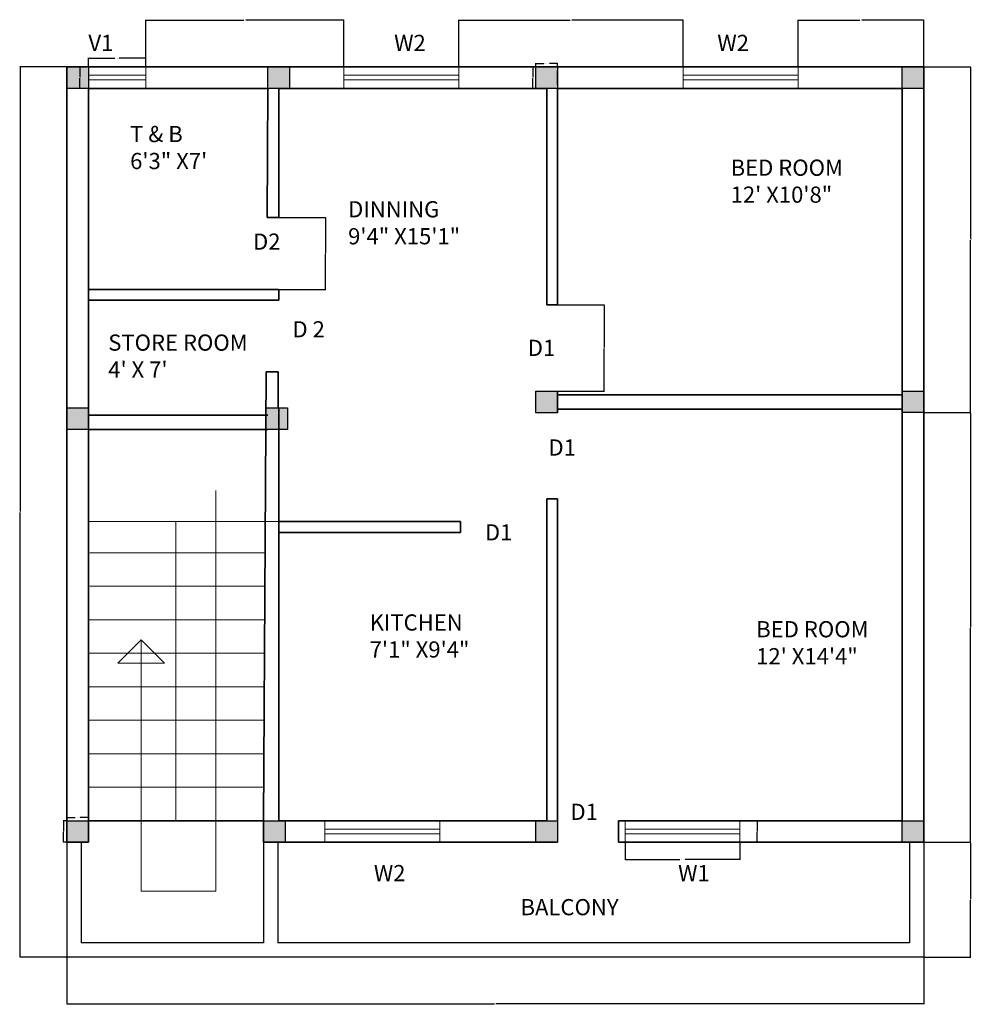
# Model space of a CAD drawing. Units: inches. Extents: x 3504 to 4623, y 2365 to 3357.
# Tile 1 of 5: x 3508 to 3905, y 2372 to 2783. Entities that reach past the tile are written whole.
import ezdxf

# ---------------------------------------------------------------- set-up
doc = ezdxf.new("R2010")
doc.units = ezdxf.units.IN
for name, color, linetype, lineweight in [('A-ANNO-DIMS', 2, 'Continuous', 18), ('A-ANNO-SYMB', 150, 'Continuous', 18), ('A-ANNO-TEXT', 7, 'Continuous', 18), ('A-AREA-IDEN', 7, 'Continuous', 18), ('A-FLOR-HRAL', 7, 'Continuous', 25), ('A-FLOR-STRS', 7, 'Continuous', 18), ('A-GLAZ', 4, 'Continuous', 18), ('A-WALL', 7, 'Continuous', 35)]:
    doc.layers.add(name, color=color, linetype=linetype, lineweight=lineweight)
doc.layers.add('S-COLS', color=244, linetype='Continuous', lineweight=30, true_color=0x991b1e)
doc.layers.add('S-COLS-PATT', color=244, linetype='Continuous', lineweight=13, true_color=0x991b1e)
doc.styles.get("Standard").update_dxf_attribs({"font": 'arial.ttf'})
doc.dimstyles.get("Standard").update_dxf_attribs({"dimtxt": 0.18, "dimasz": 0.18, "dimexe": 0.18, "dimexo": 0.0625, "dimgap": 0.09, "dimtad": 0, "dimtih": 1, "dimtoh": 1, "dimdec": 4, "dimzin": 0, "dimdsep": 46, "dimtxsty": 'Standard', "dimcen": 0.09, "dimadec": 0, "dimazin": 0, "dimtfac": 1, "dimtdec": 4, "dimtofl": 0, "dimtmove": 0, "dimatfit": 3, "dimfxl": 1, "dimtolj": 1, "dimtzin": 0, "dimarcsym": 0})

# ---------------------------------------------------------------- blocks, each defined once
blk = doc.blocks.new('WIN-48-PLAN')
for p, q in [((48, 5.5), (0, 5.5)), ((48, 3.5), (0, 3.5)), ((48, 3.5), (0, 3.5))]:
    blk.add_line(p, q)
blk.add_lwpolyline([(48, 9), (48, 0), (0, 0), (0, 9)], close=True)
blk = doc.blocks.new('VENT-24-PLAN')
for p, q in [((0, 0), (0, 9)), ((0, 9), (24, 9)), ((24, 9), (24, 0)), ((24, 5.5), (0, 5.5)), ((24, 3.5), (0, 3.5)), ((24, 3.5), (0, 3.5)), ((24, 0), (0, 0))]:
    blk.add_line(p, q)
blk = doc.blocks.new('COL-9-SQUARE')
h = blk.add_hatch(color=256)
h.dxf.hatch_style = 1
h.paths.add_polyline_path([(9, 9), (0, 9), (0, 0), (9, 0)])
blk.add_lwpolyline([(0, 9), (9, 9), (9, 0), (0, 0)], close=True)
blk = doc.blocks.new('COL-9-PERIMETER')
h = blk.add_hatch(color=256)
h.dxf.hatch_style = 1
h.paths.add_polyline_path([(9, 9), (0, 9), (0, 0), (9, 0)])
for p, q in [((0, 9), (9, 9)), ((0, 0), (0, 9)), ((9, 9), (9, 0)), ((9, 0), (0, 0))]:
    blk.add_line(p, q)
blk = doc.blocks.new('COL-9-PARTITION-HEAD')
h = blk.add_hatch(color=256)
h.dxf.hatch_style = 1
h.paths.add_polyline_path([(9, 9), (0, 9), (0, 4.5), (0, 0), (9, 0)])
blk.add_line((9, 1.5), (9, 7.5))
blk.add_lwpolyline([(0, 9), (9, 9), (9, 0), (0, 0), (0, 4.5)], close=True)
blk = doc.blocks.new('*D9')
at = {"layer": 'A-ANNO-DIMS', "color": 0, "lineweight": -2, "transparency": 16777216}
for p, q in [((3527.5, 2448.42), (3527.5, 2449.89)), ((3527.68, 2449.71), (3530.96, 2449.71)), ((3536.32, 2449.71), (3533.03, 2449.71)), ((3536.5, 2448.42), (3536.5, 2449.89))]:
    blk.add_line(p, q, dxfattribs=at)
at = {"layer": 'A-ANNO-DIMS', "color": 0, "transparency": 16777216}
for points in [[(3527.68, 2449.74), (3527.68, 2449.68), (3527.5, 2449.71)], [(3536.32, 2449.74), (3536.32, 2449.68), (3536.5, 2449.71)]]:
    blk.add_solid(points, dxfattribs=at)
at = {"layer": 'Defpoints', "color": 0, "transparency": 16777216}
for p in [(3527.5, 2448.36), (3536.5, 2449.71), (3536.5, 2448.36)]:
    blk.add_point(p, dxfattribs=at)
at = {"layer": 'A-ANNO-DIMS', "color": 0, "transparency": 16777216, "insert": (3532, 2449.71), "char_height": 0.18, "attachment_point": 5}
blk.add_mtext('\\A1;COLUMN 9 TYP.', dxfattribs=at)
blk = doc.blocks.new('*D10')
at = {"layer": 'A-ANNO-DIMS', "color": 0, "lineweight": -2, "transparency": 16777216}
for p, q in [((3527.43, 2448.36), (3525.97, 2448.36)), ((3526.15, 2448.18), (3526.15, 2444.04)), ((3526.15, 2439.54), (3526.15, 2443.68)), ((3527.43, 2439.36), (3525.97, 2439.36))]:
    blk.add_line(p, q, dxfattribs=at)
at = {"layer": 'A-ANNO-DIMS', "color": 0, "transparency": 16777216}
for points in [[(3526.12, 2448.18), (3526.18, 2448.18), (3526.15, 2448.36)], [(3526.12, 2439.54), (3526.18, 2439.54), (3526.15, 2439.36)]]:
    blk.add_solid(points, dxfattribs=at)
at = {"layer": 'Defpoints', "color": 0, "transparency": 16777216}
for p in [(3526.15, 2448.36), (3527.5, 2448.36), (3527.5, 2439.36)]:
    blk.add_point(p, dxfattribs=at)
at = {"layer": 'A-ANNO-DIMS', "color": 0, "transparency": 16777216, "insert": (3526.15, 2443.86), "char_height": 0.18, "attachment_point": 5}
blk.add_mtext('\\A1;9 TYP.', dxfattribs=at)
blk = doc.blocks.new('*D11')
at = {"layer": 'A-ANNO-DIMS', "color": 0, "lineweight": -2, "transparency": 16777216}
for p, q in [((3760.69, 2439.3), (3760.69, 2431.98)), ((3808.69, 2439.3), (3808.69, 2431.98)), ((3760.87, 2432.16), (3783.58, 2432.16)), ((3808.51, 2432.16), (3785.81, 2432.16))]:
    blk.add_line(p, q, dxfattribs=at)
at = {"layer": 'A-ANNO-DIMS', "color": 0, "transparency": 16777216}
for points in [[(3760.87, 2432.19), (3760.87, 2432.13), (3760.69, 2432.16)], [(3808.51, 2432.19), (3808.51, 2432.13), (3808.69, 2432.16)]]:
    blk.add_solid(points, dxfattribs=at)
at = {"layer": 'Defpoints', "color": 0, "transparency": 16777216}
for p in [(3760.69, 2439.36), (3808.69, 2439.36), (3808.69, 2432.16)]:
    blk.add_point(p, dxfattribs=at)
at = {"layer": 'A-ANNO-DIMS', "color": 0, "transparency": 16777216, "insert": (3784.69, 2432.16), "char_height": 0.18, "attachment_point": 5}
blk.add_mtext('\\A1;WINDOW 48 TYP.', dxfattribs=at)
blk = doc.blocks.new('*D12')
at = {"layer": 'A-ANNO-DIMS', "color": 0, "lineweight": -2, "transparency": 16777216}
for p, q in [((3808.76, 2448.36), (3816.07, 2448.36)), ((3815.89, 2448.18), (3815.89, 2444.04)), ((3815.89, 2439.54), (3815.89, 2443.68)), ((3808.76, 2439.36), (3816.07, 2439.36))]:
    blk.add_line(p, q, dxfattribs=at)
at = {"layer": 'A-ANNO-DIMS', "color": 0, "transparency": 16777216}
for points in [[(3815.86, 2448.18), (3815.92, 2448.18), (3815.89, 2448.36)], [(3815.86, 2439.54), (3815.92, 2439.54), (3815.89, 2439.36)]]:
    blk.add_solid(points, dxfattribs=at)
at = {"layer": 'Defpoints', "color": 0, "transparency": 16777216}
for p in [(3808.69, 2448.36), (3815.89, 2448.36), (3808.69, 2439.36)]:
    blk.add_point(p, dxfattribs=at)
at = {"layer": 'A-ANNO-DIMS', "color": 0, "transparency": 16777216, "insert": (3815.89, 2443.86), "char_height": 0.18, "attachment_point": 5}
blk.add_mtext('\\A1;9 TYP.', dxfattribs=at)
blk = doc.blocks.new('*D15')
at = {"layer": 'A-ANNO-DIMS', "color": 0, "lineweight": -2, "transparency": 16777216}
for p, q in [((3536.5, 2763.42), (3536.5, 2767.14)), ((3536.68, 2766.96), (3547.59, 2766.96)), ((3560.32, 2766.96), (3549.4, 2766.96)), ((3560.5, 2763.42), (3560.5, 2767.14))]:
    blk.add_line(p, q, dxfattribs=at)
at = {"layer": 'A-ANNO-DIMS', "color": 0, "transparency": 16777216}
for points in [[(3536.68, 2766.99), (3536.68, 2766.93), (3536.5, 2766.96)], [(3560.32, 2766.99), (3560.32, 2766.93), (3560.5, 2766.96)]]:
    blk.add_solid(points, dxfattribs=at)
at = {"layer": 'Defpoints', "color": 0, "transparency": 16777216}
for p in [(3560.5, 2766.96), (3536.5, 2763.36), (3560.5, 2763.36)]:
    blk.add_point(p, dxfattribs=at)
at = {"layer": 'A-ANNO-DIMS', "color": 0, "transparency": 16777216, "insert": (3548.5, 2766.96), "char_height": 0.18, "attachment_point": 5}
blk.add_mtext('\\A1;VENT 24 TYP.', dxfattribs=at)
blk = doc.blocks.new('*D16')
at = {"layer": 'A-ANNO-DIMS', "color": 0, "lineweight": -2, "transparency": 16777216}
for p, q in [((3536.43, 2763.36), (3532.72, 2763.36)), ((3532.9, 2763.18), (3532.9, 2759.04)), ((3532.9, 2754.54), (3532.9, 2758.68)), ((3536.43, 2754.36), (3532.72, 2754.36))]:
    blk.add_line(p, q, dxfattribs=at)
at = {"layer": 'A-ANNO-DIMS', "color": 0, "transparency": 16777216}
for points in [[(3532.87, 2763.18), (3532.93, 2763.18), (3532.9, 2763.36)], [(3532.87, 2754.54), (3532.93, 2754.54), (3532.9, 2754.36)]]:
    blk.add_solid(points, dxfattribs=at)
at = {"layer": 'Defpoints', "color": 0, "transparency": 16777216}
for p in [(3532.9, 2763.36), (3536.5, 2763.36), (3536.5, 2754.36)]:
    blk.add_point(p, dxfattribs=at)
at = {"layer": 'A-ANNO-DIMS', "color": 0, "transparency": 16777216, "insert": (3532.9, 2758.86), "char_height": 0.18, "attachment_point": 5}
blk.add_mtext('\\A1;9 TYP.', dxfattribs=at)
blk = doc.blocks.new('*D17')
at = {"layer": 'A-ANNO-DIMS', "color": 0, "lineweight": -2, "transparency": 16777216}
for p, q in [((3723.5, 2763.42), (3723.5, 2764.89)), ((3723.68, 2764.71), (3726.83, 2764.71)), ((3732.32, 2764.71), (3729.16, 2764.71)), ((3732.5, 2763.42), (3732.5, 2764.89))]:
    blk.add_line(p, q, dxfattribs=at)
at = {"layer": 'A-ANNO-DIMS', "color": 0, "transparency": 16777216}
for points in [[(3723.68, 2764.74), (3723.68, 2764.68), (3723.5, 2764.71)], [(3732.32, 2764.74), (3732.32, 2764.68), (3732.5, 2764.71)]]:
    blk.add_solid(points, dxfattribs=at)
at = {"layer": 'Defpoints', "color": 0, "transparency": 16777216}
for p in [(3732.5, 2764.71), (3723.5, 2763.36), (3732.5, 2763.36)]:
    blk.add_point(p, dxfattribs=at)
at = {"layer": 'A-ANNO-DIMS', "color": 0, "transparency": 16777216, "insert": (3728, 2764.71), "char_height": 0.18, "attachment_point": 5}
blk.add_mtext('\\A1;WALL COL. 9 TYP.', dxfattribs=at)
blk = doc.blocks.new('*D18')
at = {"layer": 'A-ANNO-DIMS', "color": 0, "lineweight": -2, "transparency": 16777216}
for p, q in [((3723.43, 2763.36), (3721.97, 2763.36)), ((3722.15, 2763.18), (3722.15, 2759.04)), ((3722.15, 2754.54), (3722.15, 2758.68)), ((3723.43, 2754.36), (3721.97, 2754.36))]:
    blk.add_line(p, q, dxfattribs=at)
at = {"layer": 'A-ANNO-DIMS', "color": 0, "transparency": 16777216}
for points in [[(3722.12, 2763.18), (3722.18, 2763.18), (3722.15, 2763.36)], [(3722.12, 2754.54), (3722.18, 2754.54), (3722.15, 2754.36)]]:
    blk.add_solid(points, dxfattribs=at)
at = {"layer": 'Defpoints', "color": 0, "transparency": 16777216}
for p in [(3722.15, 2763.36), (3723.5, 2763.36), (3723.5, 2754.36)]:
    blk.add_point(p, dxfattribs=at)
at = {"layer": 'A-ANNO-DIMS', "color": 0, "transparency": 16777216, "insert": (3722.15, 2758.86), "char_height": 0.18, "attachment_point": 5}
blk.add_mtext('\\A1;9 TYP.', dxfattribs=at)
blk = doc.blocks.new('*D25')
at = {"layer": 'A-ANNO-DIMS', "color": 0, "lineweight": -2, "transparency": 16777216}
for p, q in [((3527.5, 2391.3), (3527.5, 2371.68)), ((3885.5, 2391.3), (3885.5, 2371.68)), ((3527.68, 2371.86), (3706.21, 2371.86)), ((3885.32, 2371.86), (3706.79, 2371.86))]:
    blk.add_line(p, q, dxfattribs=at)
at = {"layer": 'A-ANNO-DIMS', "color": 0, "transparency": 16777216}
for points in [[(3527.68, 2371.89), (3527.68, 2371.83), (3527.5, 2371.86)], [(3885.32, 2371.89), (3885.32, 2371.83), (3885.5, 2371.86)]]:
    blk.add_solid(points, dxfattribs=at)
at = {"layer": 'Defpoints', "color": 0, "transparency": 16777216}
for p in [(3527.5, 2391.36), (3885.5, 2391.36), (3885.5, 2371.86)]:
    blk.add_point(p, dxfattribs=at)
at = {"layer": 'A-ANNO-DIMS', "color": 0, "transparency": 16777216, "insert": (3706.5, 2371.86), "char_height": 0.18, "attachment_point": 5}
blk.add_mtext('\\A1;358', dxfattribs=at)
blk = doc.blocks.new('*D26')
at = {"layer": 'A-ANNO-DIMS', "color": 0, "lineweight": -2, "transparency": 16777216}
for p, q in [((3527.43, 2763.36), (3507.82, 2763.36)), ((3508, 2763.18), (3508, 2577.54)), ((3508, 2391.54), (3508, 2577.18)), ((3527.43, 2391.36), (3507.82, 2391.36))]:
    blk.add_line(p, q, dxfattribs=at)
at = {"layer": 'A-ANNO-DIMS', "color": 0, "transparency": 16777216}
for points in [[(3507.97, 2763.18), (3508.03, 2763.18), (3508, 2763.36)], [(3507.97, 2391.54), (3508.03, 2391.54), (3508, 2391.36)]]:
    blk.add_solid(points, dxfattribs=at)
at = {"layer": 'Defpoints', "color": 0, "transparency": 16777216}
for p in [(3508, 2763.36), (3527.5, 2763.36), (3527.5, 2391.36)]:
    blk.add_point(p, dxfattribs=at)
at = {"layer": 'A-ANNO-DIMS', "color": 0, "transparency": 16777216, "insert": (3508, 2577.36), "char_height": 0.18, "attachment_point": 5}
blk.add_mtext('\\A1;372', dxfattribs=at)
blk = doc.blocks.new('*D27')
at = {"layer": 'A-ANNO-DIMS', "color": 0, "lineweight": -2, "transparency": 16777216}
for p, q in [((3885.56, 2439.36), (3905.18, 2439.36)), ((3905, 2439.18), (3905, 2415.54)), ((3905, 2391.54), (3905, 2415.18)), ((3885.56, 2391.36), (3905.18, 2391.36))]:
    blk.add_line(p, q, dxfattribs=at)
at = {"layer": 'A-ANNO-DIMS', "color": 0, "transparency": 16777216}
for points in [[(3904.97, 2439.18), (3905.03, 2439.18), (3905, 2439.36)], [(3904.97, 2391.54), (3905.03, 2391.54), (3905, 2391.36)]]:
    blk.add_solid(points, dxfattribs=at)
at = {"layer": 'Defpoints', "color": 0, "transparency": 16777216}
for p in [(3885.5, 2439.36), (3905, 2439.36), (3885.5, 2391.36)]:
    blk.add_point(p, dxfattribs=at)
at = {"layer": 'A-ANNO-DIMS', "color": 0, "transparency": 16777216, "insert": (3905, 2415.36), "char_height": 0.18, "attachment_point": 5}
blk.add_mtext('\\A1;48', dxfattribs=at)
blk = doc.blocks.new('*D28')
at = {"layer": 'A-ANNO-DIMS', "color": 0, "lineweight": -2, "transparency": 16777216}
for p, q in [((3885.56, 2618.88), (3905.18, 2618.88)), ((3905, 2618.7), (3905, 2529.3)), ((3905, 2439.54), (3905, 2528.94)), ((3885.56, 2439.36), (3905.18, 2439.36))]:
    blk.add_line(p, q, dxfattribs=at)
at = {"layer": 'A-ANNO-DIMS', "color": 0, "transparency": 16777216}
for points in [[(3904.97, 2618.7), (3905.03, 2618.7), (3905, 2618.88)], [(3904.97, 2439.54), (3905.03, 2439.54), (3905, 2439.36)]]:
    blk.add_solid(points, dxfattribs=at)
at = {"layer": 'Defpoints', "color": 0, "transparency": 16777216}
for p in [(3885.5, 2618.88), (3905, 2618.88), (3885.5, 2439.36)]:
    blk.add_point(p, dxfattribs=at)
at = {"layer": 'A-ANNO-DIMS', "color": 0, "transparency": 16777216, "insert": (3905, 2529.12), "char_height": 0.18, "attachment_point": 5}
blk.add_mtext('\\A1;179.52', dxfattribs=at)
blk = doc.blocks.new('*D29')
at = {"layer": 'A-ANNO-DIMS', "color": 0, "lineweight": -2, "transparency": 16777216}
for p, q in [((3885.56, 2763.36), (3905.18, 2763.36)), ((3905, 2763.18), (3905, 2691.3)), ((3905, 2619.06), (3905, 2690.94)), ((3885.56, 2618.88), (3905.18, 2618.88))]:
    blk.add_line(p, q, dxfattribs=at)
at = {"layer": 'A-ANNO-DIMS', "color": 0, "transparency": 16777216}
for points in [[(3904.97, 2763.18), (3905.03, 2763.18), (3905, 2763.36)], [(3904.97, 2619.06), (3905.03, 2619.06), (3905, 2618.88)]]:
    blk.add_solid(points, dxfattribs=at)
at = {"layer": 'Defpoints', "color": 0, "transparency": 16777216}
for p in [(3885.5, 2763.36), (3905, 2763.36), (3885.5, 2618.88)]:
    blk.add_point(p, dxfattribs=at)
at = {"layer": 'A-ANNO-DIMS', "color": 0, "transparency": 16777216, "insert": (3905, 2691.12), "char_height": 0.18, "attachment_point": 5}
blk.add_mtext('\\A1;144.48', dxfattribs=at)
blk = doc.blocks.new('*D30')
at = {"layer": 'A-ANNO-DIMS', "color": 0, "lineweight": -2, "transparency": 16777216}
for p, q in [((3560.5, 2763.42), (3560.5, 2783.04)), ((3560.68, 2782.86), (3601.49, 2782.86)), ((3643.09, 2782.86), (3602.27, 2782.86)), ((3643.27, 2763.42), (3643.27, 2783.04))]:
    blk.add_line(p, q, dxfattribs=at)
at = {"layer": 'A-ANNO-DIMS', "color": 0, "transparency": 16777216}
for points in [[(3560.68, 2782.89), (3560.68, 2782.83), (3560.5, 2782.86)], [(3643.09, 2782.89), (3643.09, 2782.83), (3643.27, 2782.86)]]:
    blk.add_solid(points, dxfattribs=at)
at = {"layer": 'Defpoints', "color": 0, "transparency": 16777216}
for p in [(3643.27, 2782.86), (3560.5, 2763.36), (3643.27, 2763.36)]:
    blk.add_point(p, dxfattribs=at)
at = {"layer": 'A-ANNO-DIMS', "color": 0, "transparency": 16777216, "insert": (3601.88, 2782.86), "char_height": 0.18, "attachment_point": 5}
blk.add_mtext('\\A1;82.77', dxfattribs=at)
blk = doc.blocks.new('*D31')
at = {"layer": 'A-ANNO-DIMS', "color": 0, "lineweight": -2, "transparency": 16777216}
for p, q in [((3691.27, 2763.42), (3691.27, 2783.04)), ((3691.45, 2782.86), (3737.74, 2782.86)), ((3784.83, 2782.86), (3738.53, 2782.86)), ((3785.01, 2763.42), (3785.01, 2783.04))]:
    blk.add_line(p, q, dxfattribs=at)
at = {"layer": 'A-ANNO-DIMS', "color": 0, "transparency": 16777216}
for points in [[(3691.45, 2782.89), (3691.45, 2782.83), (3691.27, 2782.86)], [(3784.83, 2782.89), (3784.83, 2782.83), (3785.01, 2782.86)]]:
    blk.add_solid(points, dxfattribs=at)
at = {"layer": 'Defpoints', "color": 0, "transparency": 16777216}
for p in [(3785.01, 2782.86), (3691.27, 2763.36), (3785.01, 2763.36)]:
    blk.add_point(p, dxfattribs=at)
at = {"layer": 'A-ANNO-DIMS', "color": 0, "transparency": 16777216, "insert": (3738.14, 2782.86), "char_height": 0.18, "attachment_point": 5}
blk.add_mtext('\\A1;93.74', dxfattribs=at)
blk = doc.blocks.new('*D32')
at = {"layer": 'A-ANNO-DIMS', "color": 0, "lineweight": -2, "transparency": 16777216}
for p, q in [((3833.01, 2763.42), (3833.01, 2783.04)), ((3833.19, 2782.86), (3858.86, 2782.86)), ((3885.32, 2782.86), (3859.65, 2782.86)), ((3885.5, 2763.42), (3885.5, 2783.04))]:
    blk.add_line(p, q, dxfattribs=at)
at = {"layer": 'A-ANNO-DIMS', "color": 0, "transparency": 16777216}
for points in [[(3833.19, 2782.89), (3833.19, 2782.83), (3833.01, 2782.86)], [(3885.32, 2782.89), (3885.32, 2782.83), (3885.5, 2782.86)]]:
    blk.add_solid(points, dxfattribs=at)
at = {"layer": 'Defpoints', "color": 0, "transparency": 16777216}
for p in [(3885.5, 2782.86), (3833.01, 2763.36), (3885.5, 2763.36)]:
    blk.add_point(p, dxfattribs=at)
at = {"layer": 'A-ANNO-DIMS', "color": 0, "transparency": 16777216, "insert": (3859.25, 2782.86), "char_height": 0.18, "attachment_point": 5}
blk.add_mtext('\\A1;52.49', dxfattribs=at)
blk = doc.blocks.new('*D33')
at = {"layer": 'A-ANNO-DIMS', "color": 0, "lineweight": -2, "transparency": 16777216}
for p, q in [((3616.06, 2700.36), (3635.68, 2700.36)), ((3635.5, 2700.18), (3635.5, 2685.54)), ((3635.5, 2670.54), (3635.5, 2685.18)), ((3616.06, 2670.36), (3635.68, 2670.36))]:
    blk.add_line(p, q, dxfattribs=at)
at = {"layer": 'A-ANNO-DIMS', "color": 0, "transparency": 16777216}
for points in [[(3635.47, 2700.18), (3635.53, 2700.18), (3635.5, 2700.36)], [(3635.47, 2670.54), (3635.53, 2670.54), (3635.5, 2670.36)]]:
    blk.add_solid(points, dxfattribs=at)
at = {"layer": 'Defpoints', "color": 0, "transparency": 16777216}
for p in [(3616, 2700.36), (3616, 2670.36), (3635.5, 2670.36)]:
    blk.add_point(p, dxfattribs=at)
at = {"layer": 'A-ANNO-DIMS', "color": 0, "transparency": 16777216, "insert": (3635.5, 2685.36), "char_height": 0.18, "attachment_point": 5}
blk.add_mtext('\\A1;30', dxfattribs=at)
blk = doc.blocks.new('*D34')
at = {"layer": 'A-ANNO-DIMS', "color": 0, "lineweight": -2, "transparency": 16777216}
for p, q in [((3732.56, 2663.86), (3752.18, 2663.86)), ((3752, 2663.68), (3752, 2646.04)), ((3752, 2628.04), (3752, 2645.68)), ((3732.56, 2627.86), (3752.18, 2627.86))]:
    blk.add_line(p, q, dxfattribs=at)
at = {"layer": 'A-ANNO-DIMS', "color": 0, "transparency": 16777216}
for points in [[(3751.97, 2663.68), (3752.03, 2663.68), (3752, 2663.86)], [(3751.97, 2628.04), (3752.03, 2628.04), (3752, 2627.86)]]:
    blk.add_solid(points, dxfattribs=at)
at = {"layer": 'Defpoints', "color": 0, "transparency": 16777216}
for p in [(3732.5, 2663.86), (3732.5, 2627.86), (3752, 2627.86)]:
    blk.add_point(p, dxfattribs=at)
at = {"layer": 'A-ANNO-DIMS', "color": 0, "transparency": 16777216, "insert": (3752, 2645.86), "char_height": 0.18, "attachment_point": 5}
blk.add_mtext('\\A1;36', dxfattribs=at)

msp = doc.modelspace()

# ---------------------------------------------------------------- hatches: boundary and pattern name
at = {"layer": 'S-COLS-PATT'}
h = msp.add_hatch(color=256, dxfattribs=at)
h.dxf.hatch_style = 1
h.paths.add_polyline_path([(3732.4963, 2627.8606), (3723.4963, 2627.8606), (3723.4963, 2623.3606), (3723.4963, 2618.8606), (3732.4963, 2618.8606)])
h.paths.add_polyline_path([(3732.4963, 2448.3606), (3723.4963, 2448.3606), (3723.4963, 2443.8606), (3723.4963, 2439.3606), (3732.4963, 2439.3606)])

# ---------------------------------------------------------------- linework, layer by layer
at = {"layer": 'A-ANNO-SYMB'}
for p, q in [((3589.7273, 2586.3138), (3589.7273, 2418.8848)), ((3558.5385, 2523.9732), (3548.7397, 2514.1745)), ((3558.5385, 2418.8848), (3558.5385, 2523.9732)), ((3568.3372, 2514.1745), (3558.5385, 2523.9732)), ((3548.7397, 2514.1745), (3568.3372, 2514.1745)), ((3589.7273, 2418.8848), (3558.5385, 2418.8848))]:
    msp.add_line(p, q, dxfattribs=at)
at = {"layer": 'A-FLOR-HRAL'}
for p, q in [((3527.4963, 2439.3606), (3527.4963, 2391.3606)), ((3533.4963, 2439.3606), (3533.4963, 2397.3606)), ((3609.6665, 2439.3606), (3609.6665, 2397.3606)), ((3615.6665, 2439.3606), (3615.6665, 2397.3606)), ((3879.4963, 2439.3606), (3879.4963, 2397.3606)), ((3885.4963, 2439.3606), (3885.4963, 2391.3606)), ((3609.6665, 2397.3606), (3533.4963, 2397.3606)), ((3732.4963, 2397.3606), (3615.6665, 2397.3606)), ((3879.4963, 2397.3606), (3732.4963, 2397.3606)), ((3732.4963, 2391.3606), (3527.4963, 2391.3606)), ((3885.4963, 2391.3606), (3732.4963, 2391.3606))]:
    msp.add_line(p, q, dxfattribs=at)
at = {"layer": 'A-FLOR-STRS'}
for p, q in [((3615.9963, 2573.3606), (3536.4963, 2573.3606)), ((3536.4963, 2573.3606), (3609.6665, 2573.3606)), ((3573.0814, 2448.3606), (3573.0814, 2573.3606)), ((3537.166, 2560.3586), (3610.3362, 2560.3586)), ((3537.0823, 2546.3588), (3610.2525, 2546.3588)), ((3536.9986, 2532.3591), (3610.1688, 2532.3591)), ((3536.9148, 2518.3593), (3610.0851, 2518.3593)), ((3536.8311, 2504.3596), (3610.0014, 2504.3596)), ((3536.7474, 2490.3598), (3609.9177, 2490.3598)), ((3536.6637, 2476.3601), (3609.8339, 2476.3601)), ((3536.58, 2462.3603), (3609.7502, 2462.3603))]:
    msp.add_line(p, q, dxfattribs=at)
at = {"layer": 'A-WALL'}
for p, q in [((3885.4963, 2763.3606), (3527.4963, 2763.3606)), ((3527.4963, 2439.3606), (3527.4963, 2763.3606)), ((3885.4963, 2439.3606), (3885.4963, 2763.3606)), ((3611.4963, 2754.3606), (3536.4963, 2754.3606)), ((3536.4963, 2474.3606), (3536.4963, 2754.3606)), ((3611.1736, 2700.3894), (3611.4963, 2754.3606)), ((3727.9963, 2754.3606), (3615.9963, 2754.3606)), ((3615.9963, 2700.3606), (3615.9963, 2754.3606)), ((3727.9963, 2663.8606), (3727.9963, 2754.3606)), ((3876.4963, 2754.3606), (3732.4963, 2754.3606)), ((3732.4963, 2663.8606), (3732.4963, 2754.3606)), ((3876.4963, 2448.3606), (3876.4963, 2754.3606)), ((3615.9963, 2700.3606), (3611.1736, 2700.3894)), ((3611.4963, 2670.3606), (3536.4963, 2670.3606)), ((3610.994, 2670.3606), (3615.9963, 2670.3606)), ((3615.9963, 2665.8606), (3615.9963, 2670.3606)), ((3610.9671, 2665.8606), (3536.4963, 2665.8606)), ((3610.9671, 2665.8606), (3615.9963, 2665.8606)), ((3727.9963, 2663.8606), (3732.4963, 2663.8606)), ((3609.6665, 2448.3606), (3610.7879, 2635.8912)), ((3615.781, 2635.8614), (3610.7879, 2635.8912)), ((3615.781, 2635.8614), (3615.781, 2620.8606)), ((3876.4963, 2626.3606), (3732.4963, 2626.3606)), ((3615.9963, 2448.3606), (3615.9963, 2620.8606)), ((3611.4963, 2617.8606), (3536.4963, 2617.8606)), ((3876.4963, 2620.3606), (3732.4963, 2620.3606)), ((3611.4963, 2611.8606), (3536.4963, 2611.8606)), ((3727.9963, 2448.3606), (3727.9963, 2582.8606)), ((3727.9963, 2582.8606), (3732.4963, 2582.8606)), ((3732.4963, 2448.3606), (3732.4963, 2582.8606)), ((3691.9963, 2573.3606), (3615.9963, 2573.3606)), ((3691.9963, 2573.3606), (3691.9963, 2568.8606)), ((3691.9963, 2568.8606), (3615.9963, 2568.8606)), ((3536.4963, 2448.3606), (3536.4963, 2474.3606)), ((3536.4963, 2448.3606), (3609.6665, 2448.3606)), ((3536.4963, 2448.3606), (3536.4963, 2439.3606)), ((3609.6665, 2448.3606), (3609.6665, 2439.3606)), ((3727.9963, 2448.3606), (3615.9963, 2448.3606)), ((3876.4963, 2448.3606), (3757.9737, 2448.3606)), ((3757.9737, 2448.3606), (3757.9737, 2439.3606)), ((3533.4963, 2439.3606), (3527.4963, 2439.3606)), ((3536.4963, 2439.3606), (3533.4963, 2439.3606)), ((3732.4963, 2439.3606), (3609.6665, 2439.3606)), ((3885.4963, 2439.3606), (3757.9737, 2439.3606))]:
    msp.add_line(p, q, dxfattribs=at)
at = {"layer": 'S-COLS'}
for p, q in [((3732.4963, 2626.3606), (3732.4963, 2627.8606)), ((3732.4963, 2620.3606), (3732.4963, 2626.3606)), ((3732.4963, 2618.8606), (3732.4963, 2620.3606))]:
    msp.add_line(p, q, dxfattribs=at)
for points in [[(3723.4963, 2627.8606), (3732.4963, 2627.8606), (3732.4963, 2618.8606), (3723.4963, 2618.8606), (3723.4963, 2623.3606)], [(3723.4963, 2448.3606), (3732.4963, 2448.3606), (3732.4963, 2439.3606), (3723.4963, 2439.3606), (3723.4963, 2443.8606)]]:
    msp.add_lwpolyline(points, close=True, dxfattribs=at)

# ---------------------------------------------------------------- block references
at = {"layer": 'A-GLAZ'}
for name, p in [('VENT-24-PLAN', (3536.4963, 2754.3606)), ('WIN-48-PLAN', (3643.266, 2754.3606)), ('WIN-48-PLAN', (3785.0071, 2754.3606)), ('WIN-48-PLAN', (3635.3055, 2439.3606)), ('WIN-48-PLAN', (3760.6941, 2439.3606))]:
    msp.add_blockref(name, p, dxfattribs=at)
at = {"layer": 'S-COLS'}
for name, p in [('COL-9-SQUARE', (3527.4963, 2754.3606)), ('COL-9-SQUARE', (3611.4963, 2754.3606)), ('COL-9-PARTITION-HEAD', (3723.4963, 2754.3606)), ('COL-9-PERIMETER', (3876.4963, 2754.3606)), ('COL-9-PERIMETER', (3876.4963, 2618.8797)), ('COL-9-SQUARE', (3527.4963, 2611.8606)), ('COL-9-SQUARE', (3610.6442, 2611.8606)), ('COL-9-SQUARE', (3527.4963, 2439.3606)), ('COL-9-SQUARE', (3609.6665, 2439.3606)), ('COL-9-PERIMETER', (3876.4963, 2439.3606))]:
    msp.add_blockref(name, p, dxfattribs=at)

# ---------------------------------------------------------------- texts
at = {"layer": 'A-ANNO-TEXT', "char_height": 6.7599, "attachment_point": 1}
for s, insert in [('V1', (3536.4963, 2776.7302)), ('W2', (3664.2349, 2776.7302)), ('W2', (3799.258, 2776.7302)), ('D2', (3605.2901, 2693.6932)), ('D 2', (3621.7478, 2657.0753)), ('D1', (3720.0666, 2649.3128)), ('D1', (3728.7013, 2607.6848)), ('D1', (3702.1725, 2572.2381)), ('D1', (3737.8881, 2455.4778)), ('W2', (3655.7472, 2429.8749)), ('W1', (3782.8726, 2429.8749))]:
    msp.add_mtext_dynamic_manual_height_columns(s, width=979.683598, gutter_width=33.7995, heights=[43.6273], dxfattribs=dict(at, insert=insert))
at = {"layer": 'A-AREA-IDEN', "attachment_point": 1}
for s, insert, char_height in [('T & B \\P6\'3" X7\'', (3553.939, 2738.6463), 6.7599), ('BED ROOM \\P12\' X10\'8"', (3804.8149, 2724.5921), 6.7599), ('DINNING\\P9\'4" X15\'1"', (3645.0069, 2707.2184), 6.759897), ("STORE ROOM \\P4' X 7'", (3544.7914, 2651.5104), 6.759897), ('KITCHEN\\P7\'1" X9\'4"', (3653.9963, 2534.5796), 6.7599), ('BED ROOM\\P12\' X14\'4"', (3815.5025, 2531.7688), 6.7599), ('BALCONY', (3717.0435, 2415.6452), 6.7599)]:
    msp.add_mtext_dynamic_manual_height_columns(s, width=979.683598, gutter_width=33.7995, heights=[43.6273], dxfattribs=dict(at, insert=insert, char_height=char_height))

# ---------------------------------------------------------------- dimensions: what is measured, and where the dimension line sits
at = {"layer": 'A-ANNO-DIMS'}
for base, p1, p2, override, picture, middle in [((3643.266, 2782.8606), (3560.4963, 2763.3606), (3643.266, 2763.3606), {"dimdec": 2, "dimlfac": 1, "dimrnd": 0, "dimzin": 0, "dimdsep": 46, "dimlunit": 2}, '*D30', (3601.8811, 2782.8606)), ((3785.0071, 2782.8606), (3691.266, 2763.3606), (3785.0071, 2763.3606), {"dimdec": 2, "dimlfac": 1, "dimrnd": 0, "dimzin": 0, "dimdsep": 46, "dimlunit": 2}, '*D31', (3738.1366, 2782.8606)), ((3885.4963, 2782.8606), (3833.0071, 2763.3606), (3885.4963, 2763.3606), {"dimdec": 2, "dimlfac": 1, "dimrnd": 0, "dimzin": 0, "dimdsep": 46, "dimlunit": 2}, '*D32', (3859.2517, 2782.8606)), ((3885.4963, 2371.8606), (3527.4963, 2391.3606), (3885.4963, 2391.3606), {"dimdec": 0, "dimlfac": 1, "dimrnd": 0, "dimzin": 0, "dimdsep": 46, "dimlunit": 2}, '*D25', (3706.4963, 2371.8606))]:
    dim = msp.add_linear_dim(base=base, p1=p1, p2=p2, dimstyle='Standard', override=override, dxfattribs=at)
    dim.commit()
    dim.dimension.update_dxf_attribs({"geometry": picture, "text_midpoint": middle})
for base, p1, p2, text, picture, middle in [((3560.4963, 2766.9606), (3536.4963, 2763.3606), (3560.4963, 2763.3606), 'VENT <> TYP.', '*D15', (3548.4963, 2766.9606)), ((3732.4963, 2764.7106), (3723.4963, 2763.3606), (3732.4963, 2763.3606), 'WALL COL. <> TYP.', '*D17', (3727.9963, 2764.7106)), ((3536.4963, 2449.7106), (3527.4963, 2448.3606), (3536.4963, 2448.3606), 'COLUMN <> TYP.', '*D9', (3531.9963, 2449.7106)), ((3808.6941, 2432.1606), (3760.6941, 2439.3606), (3808.6941, 2439.3606), 'WINDOW <> TYP.', '*D11', (3784.6941, 2432.1606))]:
    dim = msp.add_linear_dim(base=base, p1=p1, p2=p2, text=text, dimstyle='Standard', override={"dimdec": 0, "dimlfac": 1, "dimrnd": 0, "dimzin": 0, "dimdsep": 46, "dimlunit": 2}, dxfattribs=at)
    dim.commit()
    dim.dimension.update_dxf_attribs({"geometry": picture, "text_midpoint": middle})
for base, p1, p2, angle, override, picture, middle in [((3507.9963, 2763.3606), (3527.4963, 2391.3606), (3527.4963, 2763.3606), 90, {"dimdec": 0, "dimlfac": 1, "dimrnd": 0, "dimzin": 0, "dimdsep": 46, "dimlunit": 2}, '*D26', (3507.9963, 2577.3606)), ((3904.9963, 2763.3606), (3885.4963, 2618.8797), (3885.4963, 2763.3606), 90, {"dimdec": 2, "dimlfac": 1, "dimrnd": 0, "dimzin": 0, "dimdsep": 46, "dimlunit": 2}, '*D29', (3904.9963, 2691.1202)), ((3635.4963, 2670.3606), (3615.9963, 2700.3606), (3615.9963, 2670.3606), 270, {"dimdec": 0, "dimlfac": 1, "dimrnd": 0, "dimzin": 0, "dimdsep": 46, "dimlunit": 2}, '*D33', (3635.4963, 2685.3606)), ((3751.9963, 2627.8606), (3732.4963, 2663.8606), (3732.4963, 2627.8606), 270, {"dimdec": 0, "dimlfac": 1, "dimrnd": 0, "dimzin": 0, "dimdsep": 46, "dimlunit": 2}, '*D34', (3751.9963, 2645.8606)), ((3904.9963, 2618.8797), (3885.4963, 2439.3606), (3885.4963, 2618.8797), 90, {"dimdec": 2, "dimlfac": 1, "dimrnd": 0, "dimzin": 0, "dimdsep": 46, "dimlunit": 2}, '*D28', (3904.9963, 2529.1202)), ((3904.9963, 2439.3606), (3885.4963, 2391.3606), (3885.4963, 2439.3606), 90, {"dimdec": 0, "dimlfac": 1, "dimrnd": 0, "dimzin": 0, "dimdsep": 46, "dimlunit": 2}, '*D27', (3904.9963, 2415.3606))]:
    dim = msp.add_linear_dim(base=base, p1=p1, p2=p2, angle=angle, dimstyle='Standard', override=override, dxfattribs=at)
    dim.commit()
    dim.dimension.update_dxf_attribs({"geometry": picture, "text_midpoint": middle})
for base, p1, p2, picture, middle in [((3532.8963, 2763.3606), (3536.4963, 2754.3606), (3536.4963, 2763.3606), '*D16', (3532.8963, 2758.8606)), ((3722.1463, 2763.3606), (3723.4963, 2754.3606), (3723.4963, 2763.3606), '*D18', (3722.1463, 2758.8606)), ((3526.1463, 2448.3606), (3527.4963, 2439.3606), (3527.4963, 2448.3606), '*D10', (3526.1463, 2443.8606)), ((3815.8941, 2448.3606), (3808.6941, 2439.3606), (3808.6941, 2448.3606), '*D12', (3815.8941, 2443.8606))]:
    dim = msp.add_linear_dim(base=base, p1=p1, p2=p2, angle=90, text='<> TYP.', dimstyle='Standard', override={"dimdec": 0, "dimlfac": 1, "dimrnd": 0, "dimzin": 0, "dimdsep": 46, "dimlunit": 2}, dxfattribs=at)
    dim.commit()
    dim.dimension.update_dxf_attribs({"geometry": picture, "text_midpoint": middle})

doc.saveas('drawing.dxf')
